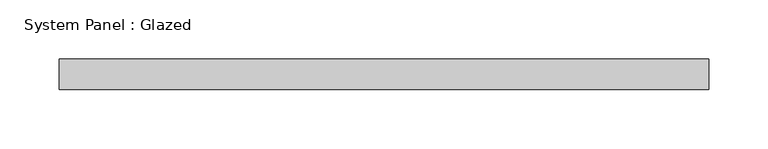
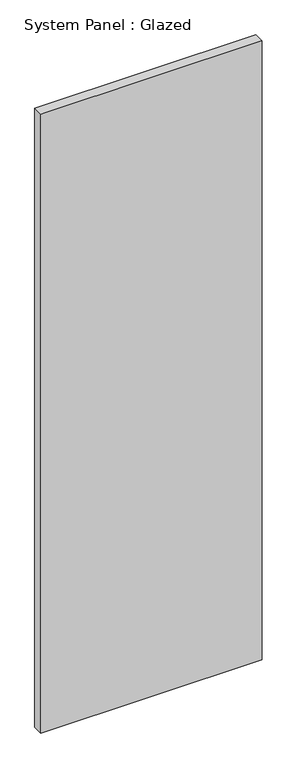
"""IFC4 building model written with IfcOpenShell, lengths in millimetres: plate geometry, System Panel : Glazed."""

from ifc_helpers import new_model, si_unit, origin, origin_with_axes, place, context, project, spatial, polyline, outline, extrude, source, transform, mapped, element, save


def system_panel_glazed_ced102d0(model_context):
    return source(origin(), model_context, "Body", "SweptSolid", [
        extrude(outline(polyline([(273.05, 19.05), (-273.05, 19.05), (-273.05, 44.45), (273.05, 44.45), (273.05, 19.05)])), origin_with_axes(), (0.0, 0.0, 1.0), 1614.7653418),
    ])


if __name__ == "__main__":
    model = new_model("IFC4")
    model_context = context("Model", 3, world=origin())
    ifc_project = project(units=[si_unit("LENGTHUNIT", "METRE", prefix="MILLI")], contexts=[model_context])
    site = spatial("IfcSite", under=ifc_project)
    building = spatial("IfcBuilding", under=site)
    placement = place(None, origin())
    system_panel_glazed_shape = system_panel_glazed_ced102d0(model_context)
    element("IfcPlate", 1, ObjectType="System Panel : Glazed", at=placement, inside=building, context=model_context, shape_type="MappedRepresentation", body=[
        mapped(system_panel_glazed_shape, transform((0.0, 0.0, 0.0), x_axis=(1.0, 0.0, 0.0), y_axis=(0.0, 1.0, 0.0), z_axis=(0.0, 0.0, 1.0))),
    ])
    save(model, "model.ifc")

# Revit data of these elements
# Type "System Panel : Glazed"
#   Construction Type Id = "GSP4R"
#   Analytic Construction = "1/8 in Pilkington single glazing"
#   Visual Light Transmittance = 0.9
#   Solar Heat Gain Coefficient = 0.86
#   Heat Transfer Coefficient (U) = 1.18115 BTU/(h·ft²·°F)
#   Define Thermal Properties by = 1
# Element 1 (IfcPlate, "System Panel : Glazed")
#   Materials on its faces: "Glass"
# Materials
#   "Glass": class "Glass", colour RGB 0 128 192, transparency 0.75, Description = "Soda Lime Glass", Cost = 0
